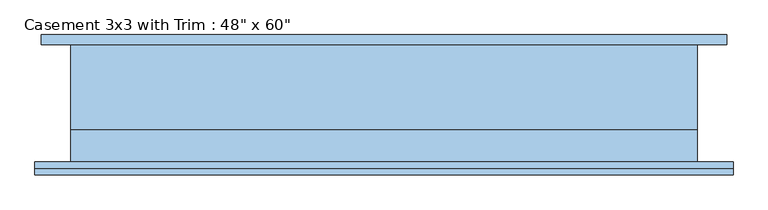
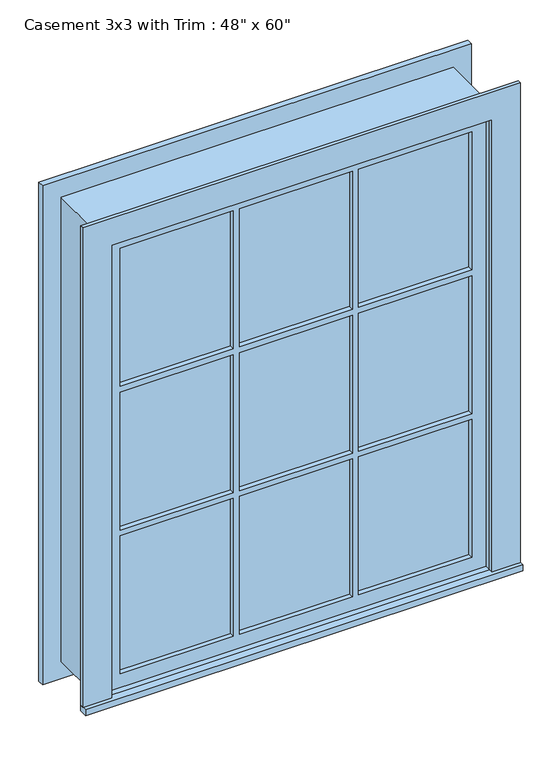
"""IFC4 building model written with IfcOpenShell, lengths in millimetres: window geometry."""

from ifc_helpers import new_model, si_unit, frame, origin, place, context, project, spatial, polyline, outline, extrude, source, transform, mapped, element, save


def window_d86b664e(model_context):
    return source(origin(), model_context, "Body", "SweptSolid", [
        extrude(outline(polyline([(-679.45, -139.7), (-679.45, -114.3), (679.45, -114.3), (679.45, -139.7), (-679.45, -139.7)])), frame((0.0, 0.0, 304.8), z_axis=(0.0, 0.0, 1.0), x_axis=(1.0, 0.0, 0.0)), (0.0, 0.0, 1.0), 19.05),
        extrude(outline(polyline([(1809.75, -590.55), (1809.75, 590.55), (323.85, 590.55), (323.85, 679.45), (1898.65, 679.45), (1898.65, -679.45), (323.85, -679.45), (323.85, -590.55), (1809.75, -590.55)])), frame((0.0, -127.0, 0.0), z_axis=(0.0, 1.0, 0.0), x_axis=(0.0, 0.0, 1.0)), (0.0, 0.0, 1.0), 12.7),
        extrude(outline(polyline([(194.7333333, -79.375), (194.7333333, -66.675), (546.1, -66.675), (546.1, -79.375), (194.7333333, -79.375)])), frame((0.0, 0.0, 1312.3333333), z_axis=(0.0, 0.0, 1.0), x_axis=(1.0, 0.0, 0.0)), (0.0, 0.0, 1.0), 452.9666667),
        extrude(outline(polyline([(-175.6833333, -79.375), (-175.6833333, -66.675), (175.6833333, -66.675), (175.6833333, -79.375), (-175.6833333, -79.375)])), frame((0.0, 0.0, 1312.3333333), z_axis=(0.0, 0.0, 1.0), x_axis=(1.0, 0.0, 0.0)), (0.0, 0.0, 1.0), 452.9666667),
        extrude(outline(polyline([(-546.1, -79.375), (-546.1, -66.675), (-194.7333333, -66.675), (-194.7333333, -79.375), (-546.1, -79.375)])), frame((0.0, 0.0, 1312.3333333), z_axis=(0.0, 0.0, 1.0), x_axis=(1.0, 0.0, 0.0)), (0.0, 0.0, 1.0), 452.9666667),
        extrude(outline(polyline([(-546.1, -79.375), (-546.1, -66.675), (-194.7333333, -66.675), (-194.7333333, -79.375), (-546.1, -79.375)])), frame((0.0, 0.0, 840.3166667), z_axis=(0.0, 0.0, 1.0), x_axis=(1.0, 0.0, 0.0)), (0.0, 0.0, 1.0), 452.9666667),
        extrude(outline(polyline([(-175.6833333, -79.375), (-175.6833333, -66.675), (175.6833333, -66.675), (175.6833333, -79.375), (-175.6833333, -79.375)])), frame((0.0, 0.0, 840.3166667), z_axis=(0.0, 0.0, 1.0), x_axis=(1.0, 0.0, 0.0)), (0.0, 0.0, 1.0), 452.9666667),
        extrude(outline(polyline([(194.7333333, -79.375), (194.7333333, -66.675), (546.1, -66.675), (546.1, -79.375), (194.7333333, -79.375)])), frame((0.0, 0.0, 840.3166667), z_axis=(0.0, 0.0, 1.0), x_axis=(1.0, 0.0, 0.0)), (0.0, 0.0, 1.0), 452.9666667),
        extrude(outline(polyline([(194.7333333, -79.375), (194.7333333, -66.675), (546.1, -66.675), (546.1, -79.375), (194.7333333, -79.375)])), frame((0.0, 0.0, 368.3), z_axis=(0.0, 0.0, 1.0), x_axis=(1.0, 0.0, 0.0)), (0.0, 0.0, 1.0), 452.9666667),
        extrude(outline(polyline([(-175.6833333, -79.375), (-175.6833333, -66.675), (175.6833333, -66.675), (175.6833333, -79.375), (-175.6833333, -79.375)])), frame((0.0, 0.0, 368.3), z_axis=(0.0, 0.0, 1.0), x_axis=(1.0, 0.0, 0.0)), (0.0, 0.0, 1.0), 452.9666667),
        extrude(outline(polyline([(-546.1, -79.375), (-546.1, -66.675), (-194.7333333, -66.675), (-194.7333333, -79.375), (-546.1, -79.375)])), frame((0.0, 0.0, 368.3), z_axis=(0.0, 0.0, 1.0), x_axis=(1.0, 0.0, 0.0)), (0.0, 0.0, 1.0), 452.9666667),
        extrude(outline(polyline([(1885.95, 666.75), (1885.95, -666.75), (247.65, -666.75), (247.65, 666.75), (1885.95, 666.75)]), holes=[polyline([(1797.05, 577.85), (336.55, 577.85), (336.55, -577.85), (1797.05, -577.85), (1797.05, 577.85)])]), frame((0.0, 114.3, 0.0), z_axis=(0.0, 1.0, 0.0), x_axis=(0.0, 0.0, 1.0)), (0.0, 0.0, 1.0), 19.05),
        extrude(outline(polyline([(1809.75, -590.55), (323.85, -590.55), (323.85, 590.55), (1809.75, 590.55), (1809.75, -590.55)]), holes=[polyline([(1765.3, -194.7333333), (1312.3333333, -194.7333333), (1312.3333333, -546.1), (1765.3, -546.1), (1765.3, -194.7333333)]), polyline([(1293.2833333, -194.7333333), (840.3166667, -194.7333333), (840.3166667, -546.1), (1293.2833333, -546.1), (1293.2833333, -194.7333333)]), polyline([(821.2666667, -194.7333333), (368.3, -194.7333333), (368.3, -546.1), (821.2666667, -546.1), (821.2666667, -194.7333333)]), polyline([(1765.3, 175.6833333), (1312.3333333, 175.6833333), (1312.3333333, -175.6833333), (1765.3, -175.6833333), (1765.3, 175.6833333)]), polyline([(1293.2833333, 175.6833333), (840.3166667, 175.6833333), (840.3166667, -175.6833333), (1293.2833333, -175.6833333), (1293.2833333, 175.6833333)]), polyline([(821.2666667, 175.6833333), (368.3, 175.6833333), (368.3, -175.6833333), (821.2666667, -175.6833333), (821.2666667, 175.6833333)]), polyline([(1765.3, 546.1), (1312.3333333, 546.1), (1312.3333333, 194.7333333), (1765.3, 194.7333333), (1765.3, 546.1)]), polyline([(1293.2833333, 546.1), (840.3166667, 546.1), (840.3166667, 194.7333333), (1293.2833333, 194.7333333), (1293.2833333, 546.1)]), polyline([(821.2666667, 546.1), (368.3, 546.1), (368.3, 194.7333333), (821.2666667, 194.7333333), (821.2666667, 546.1)])]), frame((0.0, -95.25, 0.0), z_axis=(0.0, 1.0, 0.0), x_axis=(0.0, 0.0, 1.0)), (0.0, 0.0, 1.0), 44.45),
        extrude(outline(polyline([(1828.8, -609.6), (304.8, -609.6), (304.8, 609.6), (1828.8, 609.6), (1828.8, -609.6)]), holes=[polyline([(1797.05, -577.85), (1797.05, 577.85), (336.55, 577.85), (336.55, -577.85), (1797.05, -577.85)])]), frame((0.0, -50.8, 0.0), z_axis=(0.0, 1.0, 0.0), x_axis=(0.0, 0.0, 1.0)), (0.0, 0.0, 1.0), 165.1),
        extrude(outline(polyline([(1828.8, 609.6), (1828.8, -609.6), (304.8, -609.6), (304.8, 609.6), (1828.8, 609.6)]), holes=[polyline([(1809.75, 590.55), (323.85, 590.55), (323.85, -590.55), (1809.75, -590.55), (1809.75, 590.55)])]), frame((0.0, -114.3, 0.0), z_axis=(0.0, 1.0, 0.0), x_axis=(0.0, 0.0, 1.0)), (0.0, 0.0, 1.0), 63.5),
    ])


if __name__ == "__main__":
    model = new_model("IFC4")
    model_context = context("Model", 3, world=origin())
    ifc_project = project(units=[si_unit("LENGTHUNIT", "METRE", prefix="MILLI")], contexts=[model_context])
    site = spatial("IfcSite", under=ifc_project)
    building = spatial("IfcBuilding", under=site)
    placement = place(None, origin())
    window_shape = window_d86b664e(model_context)
    element("IfcWindow", 1, ObjectType="Casement 3x3 with Trim : 48\" x 60\"", at=placement, inside=building, context=model_context, shape_type="MappedRepresentation", body=[
        mapped(window_shape, transform((0.0, 0.0, 0.0), x_axis=(1.0, 0.0, 0.0), y_axis=(0.0, 1.0, 0.0), z_axis=(0.0, 0.0, 1.0))),
    ])
    save(model, "model.ifc")

# Revit data of these elements
# Type "Casement 3x3 with Trim : 48\" x 60\""
#   Type Mark = "12"
#   Construction Type Id = "GSP4R"
#   Assembly Code = "B2020100"
#   Analytic Construction = "1/8 in Pilkington single glazing"
#   Visual Light Transmittance = 0.9
#   Solar Heat Gain Coefficient = 0.78
#   Heat Transfer Coefficient (U) = 0.6496 BTU/(h·ft²·°F)
#   Height = 5' - 0"
#   Default Sill Height = 1' - 0"
#   Trim Projection - Ext. = 0' - 0 1/2"
#   Trim Projection - Int. = 0' - 0 3/4"
#   Trim Width - Exterior = 0' - 3 1/2"
#   Trim Width - Interior = 0' - 3 1/2"
#   Width = 4' - 0"
#   Window Inset = 0' - 0 3/4"
#   Define Thermal Properties by = 1
#   Glass Pane Material = Glass
#   Sash Material = Sash
#   Trim Exterior Material = Trim
#   Trim Interior Material = Trim
#   Wall Closure = (empty or 0)
# Element 1 (IfcWindow, "Casement 3x3 with Trim : 48\" x 60\"")
#   Materials on its faces: "Sash", "Glass", "Trim"
# Materials
#   "Glass": class "Glass", colour RGB 0 128 192, transparency 0.75, Description = "Soda Lime Glass", Cost = 0
#   "Sash": class "Wood", colour RGB 224 178 126, transparency 0
#   "Trim": class "Wood", colour RGB 224 178 126, transparency 0
